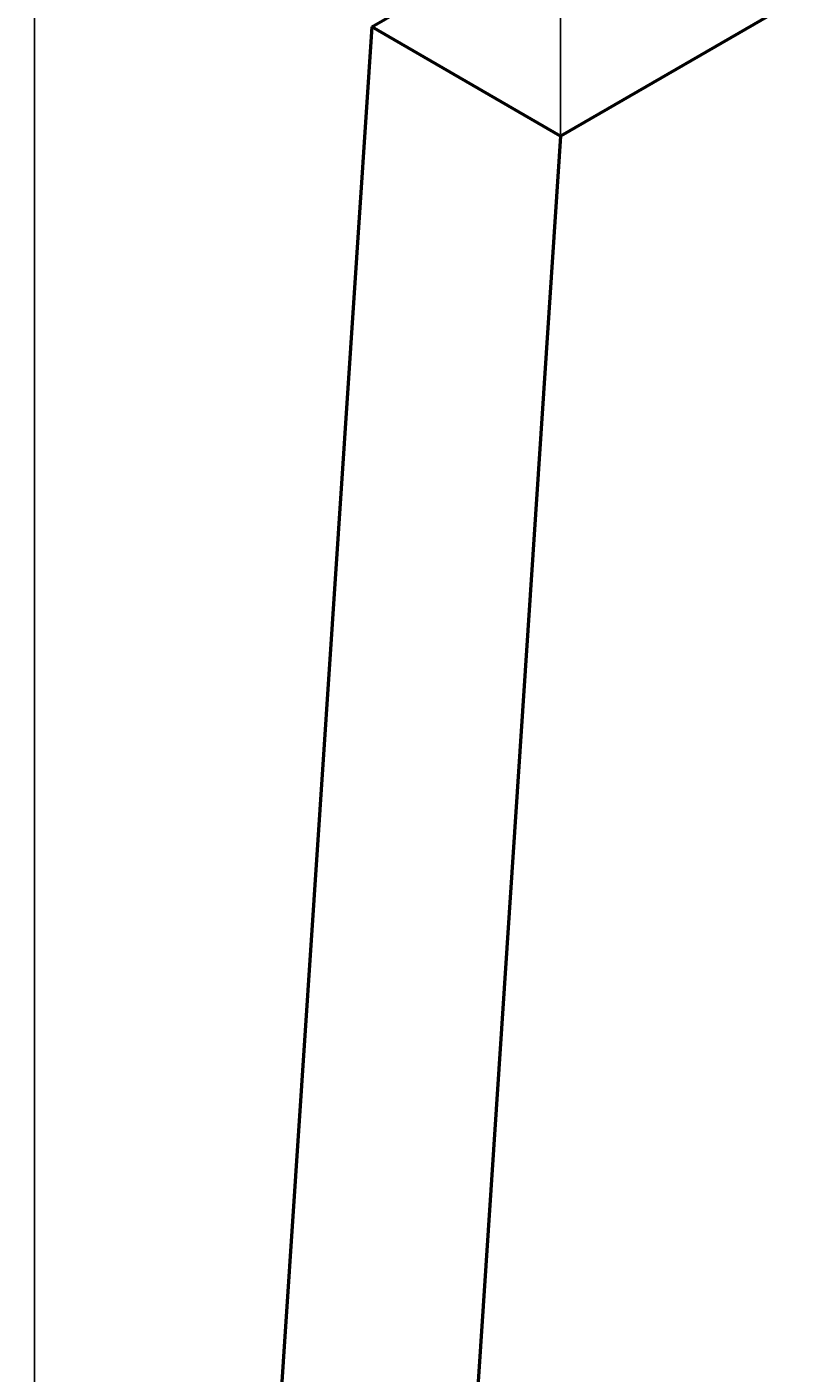
# Model space of a CAD drawing. Units: inches. Extents: x -23 to 69, y -27 to 96.
# Tile 5 of 10: x -23 to -2, y 35 to 72. Entities that reach past the tile are written whole.
import ezdxf

# ---------------------------------------------------------------- set-up
doc = ezdxf.new("R2010")
doc.units = ezdxf.units.IN
doc.header["$MEASUREMENT"] = 0
doc.layers.add('M-DIMS', color=2, linetype='Continuous', lineweight=18)
doc.layers.add('M-OUTL', color=7, linetype='Continuous', lineweight=50)
doc.styles.get("Standard").update_dxf_attribs({"font": 'arial.ttf'})
doc.dimstyles.get("Standard").update_dxf_attribs({"dimtxt": 0.18, "dimasz": 0.18, "dimexe": 0.18, "dimexo": 0.0625, "dimgap": 0.09, "dimtad": 0, "dimtih": 1, "dimtoh": 1, "dimdec": 4, "dimzin": 0, "dimdsep": 46, "dimtxsty": 'Standard', "dimcen": 0.09, "dimadec": 0, "dimazin": 0, "dimtfac": 1, "dimtdec": 4, "dimtofl": 0, "dimtmove": 0, "dimatfit": 3, "dimfxl": 1, "dimtolj": 1, "dimtzin": 0, "dimarcsym": 0})

# ---------------------------------------------------------------- blocks, each defined once
blk = doc.blocks.new('*D13')
at = {"layer": 'Defpoints', "color": 0, "transparency": 16777216}
for p in [(15.838, 89.119), (-22.888, -20.881), (36.623, -20.881)]:
    blk.add_point(p, dxfattribs=at)
at = {"layer": 'M-DIMS', "color": 0, "lineweight": -2, "transparency": 16777216}
for p, q in [((15.776, 89.119), (-23.068, 89.119)), ((-22.888, 88.939), (-22.888, 34.301)), ((-22.888, -20.701), (-22.888, 33.937)), ((36.56, -20.881), (-23.068, -20.881))]:
    blk.add_line(p, q, dxfattribs=at)
at = {"layer": 'M-DIMS', "color": 0, "transparency": 16777216}
for points in [[(-22.918, 88.939), (-22.858, 88.939), (-22.888, 89.119)], [(-22.918, -20.701), (-22.858, -20.701), (-22.888, -20.881)]]:
    blk.add_solid(points, dxfattribs=at)
at = {"layer": 'M-DIMS', "color": 0, "transparency": 16777216, "insert": (-22.888, 34.119), "char_height": 0.18, "attachment_point": 5}
blk.add_mtext('\\A1;110', dxfattribs=at)
blk = doc.blocks.new('*D16')
at = {"layer": 'Defpoints', "color": 0, "transparency": 16777216}
for p in [(17.57, 95.369), (-8.41, 69.119), (17.57, 52.119)]:
    blk.add_point(p, dxfattribs=at)
at = {"layer": 'M-DIMS', "color": 0, "lineweight": -2, "transparency": 16777216}
for p, q in [((-8.41, 69.181), (-8.41, 95.549)), ((17.57, 52.181), (17.57, 95.549)), ((-8.23, 95.369), (4.184, 95.369)), ((17.39, 95.369), (4.975, 95.369))]:
    blk.add_line(p, q, dxfattribs=at)
at = {"layer": 'M-DIMS', "color": 0, "transparency": 16777216}
for points in [[(-8.23, 95.399), (-8.23, 95.339), (-8.41, 95.369)], [(17.39, 95.399), (17.39, 95.339), (17.57, 95.369)]]:
    blk.add_solid(points, dxfattribs=at)
at = {"layer": 'M-DIMS', "color": 0, "transparency": 16777216, "insert": (4.58, 95.369), "char_height": 0.18, "attachment_point": 5}
blk.add_mtext('\\A1;25.98', dxfattribs=at)

msp = doc.modelspace()

# ---------------------------------------------------------------- linework, layer by layer
at = {"layer": 'M-OUTL'}
for p, q in [((-13.6066, 72.1186), (15.8382, 89.1186)), ((21.0344, 86.1186), (-8.4105, 69.1186)), ((-13.6066, 72.1186), (-16.6377, 26.3686)), ((-8.4105, 69.1186), (-13.6066, 72.1186)), ((-8.4105, 69.1186), (-11.4416, 23.3686))]:
    msp.add_line(p, q, dxfattribs=at)

# ---------------------------------------------------------------- dimensions: what is measured, and where the dimension line sits
at = {"layer": 'M-DIMS'}
dim = msp.add_linear_dim(base=(17.5703, 95.3686), p1=(-8.4105, 69.1186), p2=(17.5703, 52.1186), dimstyle='Standard', override={"dimdec": 2, "dimlfac": 1, "dimrnd": 0, "dimzin": 0, "dimdsep": 46, "dimlunit": 2}, dxfattribs=at)
dim.commit()
dim.dimension.update_dxf_attribs({"geometry": '*D16', "text_midpoint": (4.5799, 95.3686)})
dim = msp.add_linear_dim(base=(-22.8877, -20.8814), p1=(15.8382, 89.1186), p2=(36.6228, -20.8814), angle=90, dimstyle='Standard', override={"dimdec": 0, "dimlfac": 1, "dimrnd": 0, "dimzin": 0, "dimdsep": 46, "dimlunit": 2}, dxfattribs=at)
dim.commit()
dim.dimension.update_dxf_attribs({"geometry": '*D13', "text_midpoint": (-22.8877, 34.1186)})

doc.saveas('drawing.dxf')
